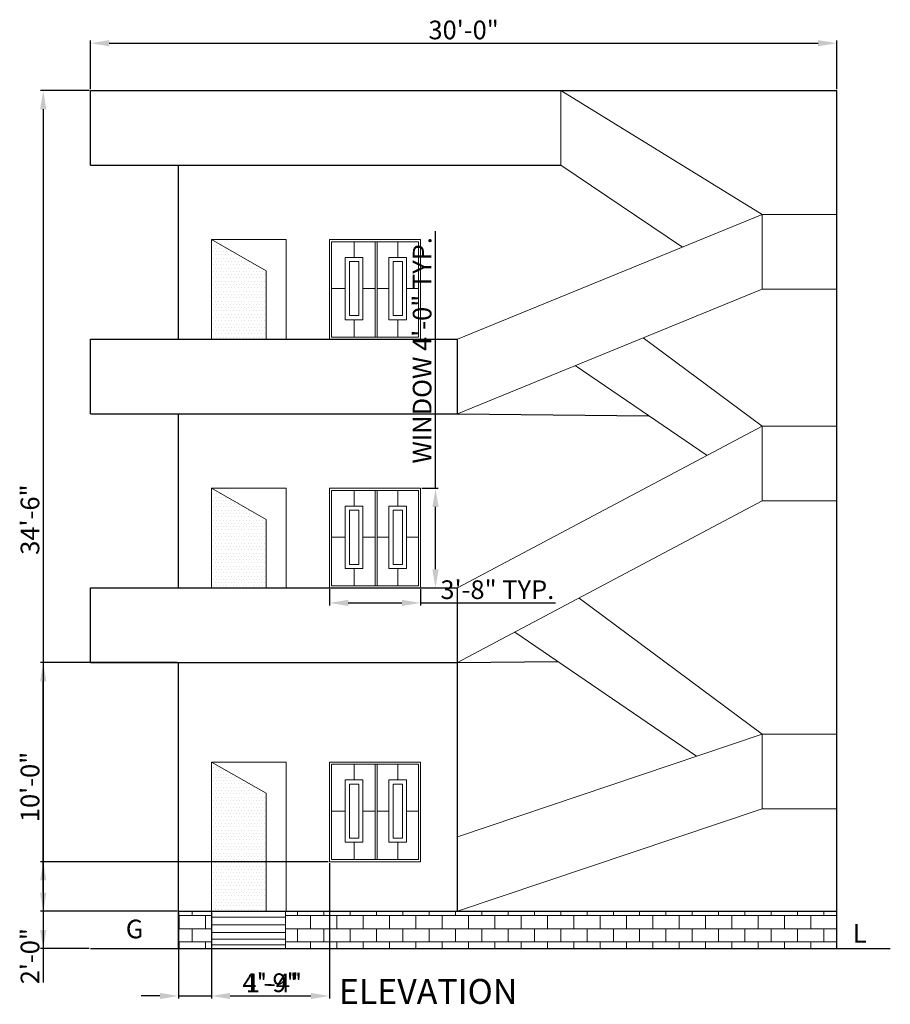
# Model space of a CAD drawing. Units: inches. Extents: x 2044 to 3644, y 808 to 1988.
# Tile 2 of 4: x 2082 to 2502, y 1513 to 1988. Entities that reach past the tile are written whole.
import ezdxf

# ---------------------------------------------------------------- set-up
doc = ezdxf.new("R2010")
doc.units = ezdxf.units.IN
for name, color, linetype, lineweight in [('A-ANNO-DIMS', 2, 'Continuous', 18), ('A-ANNO-SYMB', 2, 'Continuous', 18), ('A-ANNO-TITL', 7, 'Continuous', 25), ('A-DOOR', 4, 'Continuous', 18), ('A-DOOR-PATT', 252, 'Continuous', 13), ('A-ELEV', 7, 'Continuous', 25), ('A-FLOR-STRS', 3, 'Continuous', 18), ('A-GLAZ', 4, 'Continuous', 18), ('A-WALL-PATT', 252, 'Continuous', 13)]:
    doc.layers.add(name, color=color, linetype=linetype, lineweight=lineweight)
doc.styles.get("Standard").update_dxf_attribs({"font": 'arial.ttf'})
doc.dimstyles.new('ISO-25', dxfattribs={"dimtxt": 9, "dimasz": 9, "dimexe": 1.25, "dimexo": 0.625, "dimtad": 1, "dimdec": 1, "dimrnd": 9, "dimlunit": 3, "dimtxsty": 'Standard', "dimcen": 2.5, "dimadec": 0, "dimazin": 0, "dimtfac": 1, "dimtdec": 1, "dimtmove": 0, "dimatfit": 3, "dimfxl": 1, "dimarcsym": 0})

# ---------------------------------------------------------------- blocks, each defined once
blk = doc.blocks.new('WIN-TWIN-PANEL-ELEV')
for p, q in [((11.88, 39.49), (11.88, 47.1)), ((21.96, 47.1), (21.96, 1)), ((22.96, 47.1), (22.96, 1)), ((32.93, 39.49), (32.93, 47.1)), ((1, 24.45), (7.61, 24.45)), ((16.15, 24.45), (21.96, 24.45)), ((22.96, 24.45), (28.66, 24.45)), ((37.2, 24.45), (42.91, 24.45)), ((11.88, 9.41), (11.88, 1)), ((32.93, 9.41), (32.93, 1))]:
    blk.add_line(p, q)
for points in [[(0, 48.1), (43.91, 48.1), (43.91, 0), (0, 0)], [(1, 47.1), (42.91, 47.1), (42.91, 1), (1, 1)], [(7.61, 39.49), (16.15, 39.49), (16.15, 9.41), (7.61, 9.41)], [(28.66, 39.49), (37.2, 39.49), (37.2, 9.41), (28.66, 9.41)], [(9.61, 37.49), (14.15, 37.49), (14.15, 11.41), (9.61, 11.41)], [(30.66, 37.49), (35.2, 37.49), (35.2, 11.41), (30.66, 11.41)]]:
    blk.add_lwpolyline(points, close=True)
blk = doc.blocks.new('*D43')
at = {"layer": 'A-ANNO-DIMS', "color": 0, "lineweight": -2, "transparency": 16777216}
for p, q in [((2282.74, 1761.93), (2282.74, 1886.07)), ((2276.15, 1761.93), (2283.99, 1761.93)), ((2282.74, 1722.83), (2282.74, 1752.93)), ((2276.15, 1713.83), (2283.99, 1713.83))]:
    blk.add_line(p, q, dxfattribs=at)
at = {"layer": 'A-ANNO-DIMS', "color": 0, "transparency": 16777216}
for points in [[(2281.24, 1752.93), (2284.24, 1752.93), (2282.74, 1761.93)], [(2281.24, 1722.83), (2284.24, 1722.83), (2282.74, 1713.83)]]:
    blk.add_solid(points, dxfattribs=at)
at = {"layer": 'Defpoints', "color": 0, "transparency": 16777216}
for p in [(2275.52, 1761.93), (2282.74, 1761.93), (2275.52, 1713.83)]:
    blk.add_point(p, dxfattribs=at)
at = {"layer": 'A-ANNO-DIMS', "color": 0, "transparency": 16777216, "insert": (2277.46, 1828.5), "char_height": 9, "attachment_point": 5, "rotation": 90}
blk.add_mtext('WINDOW 4\'-0" TYP.', dxfattribs=at)
blk = doc.blocks.new('*D44')
at = {"layer": 'A-ANNO-DIMS', "color": 0, "lineweight": -2, "transparency": 16777216}
for p, q in [((2231.61, 1713.21), (2231.61, 1705.37)), ((2275.52, 1713.21), (2275.52, 1705.37)), ((2240.61, 1706.62), (2266.52, 1706.62)), ((2275.52, 1706.62), (2340.63, 1706.62))]:
    blk.add_line(p, q, dxfattribs=at)
at = {"layer": 'A-ANNO-DIMS', "color": 0, "transparency": 16777216}
for points in [[(2240.61, 1708.12), (2240.61, 1705.12), (2231.61, 1706.62)], [(2266.52, 1708.12), (2266.52, 1705.12), (2275.52, 1706.62)]]:
    blk.add_solid(points, dxfattribs=at)
at = {"layer": 'Defpoints', "color": 0, "transparency": 16777216}
for p in [(2231.61, 1713.83), (2275.52, 1713.83), (2275.52, 1706.62)]:
    blk.add_point(p, dxfattribs=at)
at = {"layer": 'A-ANNO-DIMS', "color": 0, "transparency": 16777216, "insert": (2312.58, 1711.84), "char_height": 9, "attachment_point": 5}
blk.add_mtext('3\'-8" TYP.', dxfattribs=at)
blk = doc.blocks.new('*D62')
at = {"layer": 'A-ANNO-DIMS', "color": 0, "lineweight": -2, "transparency": 16777216}
for p, q in [((2116.33, 1954.46), (2116.33, 1977.93)), ((2125.33, 1976.68), (2467.33, 1976.68)), ((2476.33, 1954.46), (2476.33, 1977.93))]:
    blk.add_line(p, q, dxfattribs=at)
at = {"layer": 'A-ANNO-DIMS', "color": 0, "transparency": 16777216}
for points in [[(2125.33, 1978.18), (2125.33, 1975.18), (2116.33, 1976.68)], [(2467.33, 1978.18), (2467.33, 1975.18), (2476.33, 1976.68)]]:
    blk.add_solid(points, dxfattribs=at)
at = {"layer": 'Defpoints', "color": 0, "transparency": 16777216}
for p in [(2476.33, 1976.68), (2116.33, 1953.83), (2476.33, 1953.83)]:
    blk.add_point(p, dxfattribs=at)
at = {"layer": 'A-ANNO-DIMS', "color": 0, "transparency": 16777216, "insert": (2296.33, 1981.91), "char_height": 9, "attachment_point": 5}
blk.add_mtext('30\'-0"', dxfattribs=at)
blk = doc.blocks.new('*D63')
at = {"layer": 'A-ANNO-DIMS', "color": 0, "lineweight": -2, "transparency": 16777216}
for p, q in [((2115.7, 1953.83), (2092.23, 1953.83)), ((2093.48, 1944.83), (2093.48, 1548.83)), ((2115.7, 1539.83), (2092.23, 1539.83))]:
    blk.add_line(p, q, dxfattribs=at)
at = {"layer": 'A-ANNO-DIMS', "color": 0, "transparency": 16777216}
for points in [[(2091.98, 1944.83), (2094.98, 1944.83), (2093.48, 1953.83)], [(2091.98, 1548.83), (2094.98, 1548.83), (2093.48, 1539.83)]]:
    blk.add_solid(points, dxfattribs=at)
at = {"layer": 'Defpoints', "color": 0, "transparency": 16777216}
for p in [(2116.33, 1953.83), (2093.48, 1539.83), (2116.33, 1539.83)]:
    blk.add_point(p, dxfattribs=at)
at = {"layer": 'A-ANNO-DIMS', "color": 0, "transparency": 16777216, "insert": (2088.25, 1746.83), "char_height": 9, "attachment_point": 5, "rotation": 90}
blk.add_mtext('34\'-6"', dxfattribs=at)
blk = doc.blocks.new('*D64')
at = {"layer": 'A-ANNO-DIMS', "color": 0, "lineweight": -2, "transparency": 16777216}
for p, q in [((2158.74, 1557.21), (2158.74, 1515.73)), ((2174.67, 1557.21), (2174.67, 1515.73)), ((2149.74, 1516.98), (2140.74, 1516.98)), ((2158.74, 1516.98), (2174.67, 1516.98)), ((2183.67, 1516.98), (2217, 1516.98))]:
    blk.add_line(p, q, dxfattribs=at)
at = {"layer": 'A-ANNO-DIMS', "color": 0, "transparency": 16777216}
for points in [[(2149.74, 1518.48), (2149.74, 1515.48), (2158.74, 1516.98)], [(2183.67, 1518.48), (2183.67, 1515.48), (2174.67, 1516.98)]]:
    blk.add_solid(points, dxfattribs=at)
at = {"layer": 'Defpoints', "color": 0, "transparency": 16777216}
for p in [(2158.74, 1557.83), (2174.67, 1557.83), (2174.67, 1516.98)]:
    blk.add_point(p, dxfattribs=at)
at = {"layer": 'A-ANNO-DIMS', "color": 0, "transparency": 16777216, "insert": (2204.84, 1522.13), "char_height": 9, "attachment_point": 5}
blk.add_mtext('1\'-4"', dxfattribs=at)
blk = doc.blocks.new('*D65')
at = {"layer": 'A-ANNO-DIMS', "color": 0, "lineweight": -2, "transparency": 16777216}
for p, q in [((2231.61, 1581.11), (2231.61, 1515.73)), ((2174.67, 1557.21), (2174.67, 1515.73)), ((2183.67, 1516.98), (2222.61, 1516.98))]:
    blk.add_line(p, q, dxfattribs=at)
at = {"layer": 'A-ANNO-DIMS', "color": 0, "transparency": 16777216}
for points in [[(2183.67, 1518.48), (2183.67, 1515.48), (2174.67, 1516.98)], [(2222.61, 1518.48), (2222.61, 1515.48), (2231.61, 1516.98)]]:
    blk.add_solid(points, dxfattribs=at)
at = {"layer": 'Defpoints', "color": 0, "transparency": 16777216}
for p in [(2231.61, 1581.74), (2174.67, 1557.83), (2231.61, 1516.98)]:
    blk.add_point(p, dxfattribs=at)
at = {"layer": 'A-ANNO-DIMS', "color": 0, "transparency": 16777216, "insert": (2203.14, 1522.2), "char_height": 9, "attachment_point": 5}
blk.add_mtext('4\'-9"', dxfattribs=at)
blk = doc.blocks.new('*D66')
at = {"layer": 'A-ANNO-DIMS', "color": 0, "lineweight": -2, "transparency": 16777216}
for p, q in [((2230.99, 1581.74), (2092.23, 1581.74)), ((2093.48, 1572.74), (2093.48, 1566.83)), ((2158.12, 1557.83), (2092.23, 1557.83)), ((2093.48, 1557.83), (2093.48, 1523.51))]:
    blk.add_line(p, q, dxfattribs=at)
at = {"layer": 'A-ANNO-DIMS', "color": 0, "transparency": 16777216}
for points in [[(2091.98, 1572.74), (2094.98, 1572.74), (2093.48, 1581.74)], [(2091.98, 1566.83), (2094.98, 1566.83), (2093.48, 1557.83)]]:
    blk.add_solid(points, dxfattribs=at)
at = {"layer": 'Defpoints', "color": 0, "transparency": 16777216}
for p in [(2231.61, 1581.74), (2093.48, 1557.83), (2158.74, 1557.83)]:
    blk.add_point(p, dxfattribs=at)
at = {"layer": 'A-ANNO-DIMS', "color": 0, "transparency": 16777216, "insert": (2088.26, 1536.17), "char_height": 9, "attachment_point": 5, "rotation": 90}
blk.add_mtext('2\'-0"', dxfattribs=at)
blk = doc.blocks.new('*D67')
at = {"layer": 'A-ANNO-DIMS', "color": 0, "lineweight": -2, "transparency": 16777216}
for p, q in [((2158.12, 1677.83), (2092.23, 1677.83)), ((2093.48, 1566.83), (2093.48, 1668.83)), ((2158.12, 1557.83), (2092.23, 1557.83))]:
    blk.add_line(p, q, dxfattribs=at)
at = {"layer": 'A-ANNO-DIMS', "color": 0, "transparency": 16777216}
for points in [[(2091.98, 1668.83), (2094.98, 1668.83), (2093.48, 1677.83)], [(2091.98, 1566.83), (2094.98, 1566.83), (2093.48, 1557.83)]]:
    blk.add_solid(points, dxfattribs=at)
at = {"layer": 'Defpoints', "color": 0, "transparency": 16777216}
for p in [(2093.48, 1677.83), (2158.74, 1677.83), (2158.74, 1557.83)]:
    blk.add_point(p, dxfattribs=at)
at = {"layer": 'A-ANNO-DIMS', "color": 0, "transparency": 16777216, "insert": (2088.26, 1617.83), "char_height": 9, "attachment_point": 5, "rotation": 90}
blk.add_mtext('10\'-0"', dxfattribs=at)

msp = doc.modelspace()

# ---------------------------------------------------------------- hatches: boundary and pattern name
at = {"layer": 'A-DOOR-PATT'}
h = msp.add_hatch(dxfattribs=at)
h.set_pattern_fill('DOTS', color=256)
h.set_pattern_definition([(0, (9e-13, 252.0964), (0.79375, 1.5875), [0, -1.5875])])
h.paths.add_polyline_path([(2174.67, 1833.83), (2201.07, 1833.83), (2201.07, 1866.86), (2174.67, 1881.93)])
h = msp.add_hatch(dxfattribs=at)
h.set_pattern_fill('DOTS', color=256)
h.set_pattern_definition([(0, (1e-12, 132.0964), (0.79375, 1.5875), [0, -1.5875])])
h.paths.add_polyline_path([(2174.67, 1713.83), (2201.07, 1713.83), (2201.07, 1746.86), (2174.67, 1761.93)])
h = msp.add_hatch(dxfattribs=at)
h.set_pattern_fill('DOTS', color=256)
h.paths.add_polyline_path([(2201.07, 1614.76), (2174.67, 1629.83), (2174.67, 1557.83), (2201.07, 1557.83)])
at = {"layer": 'A-WALL-PATT'}
h = msp.add_hatch(dxfattribs=at)
h.set_pattern_fill('BRICK', color=256)
h.paths.add_polyline_path([(2476.33, 1557.83), (2210.41, 1557.83), (2210.41, 1539.83), (2476.33, 1539.83)])
h.paths.add_polyline_path([(2174.67, 1557.83), (2158.74, 1557.83), (2158.74, 1539.83), (2174.67, 1539.83)])

# ---------------------------------------------------------------- linework, layer by layer
at = {"layer": 'A-DOOR'}
for p, q in [((2174.67, 1833.83), (2174.67, 1881.93)), ((2174.67, 1881.93), (2210.67, 1881.93)), ((2174.67, 1881.93), (2201.07, 1866.86)), ((2210.67, 1881.93), (2210.67, 1833.83)), ((2201.07, 1866.86), (2201.07, 1833.83)), ((2174.67, 1713.83), (2174.67, 1761.93)), ((2174.67, 1761.93), (2210.67, 1761.93)), ((2174.67, 1761.93), (2201.07, 1746.86)), ((2210.67, 1761.93), (2210.67, 1713.83)), ((2201.07, 1746.86), (2201.07, 1713.83)), ((2174.67, 1557.83), (2174.67, 1629.83)), ((2174.67, 1629.83), (2210.67, 1629.83)), ((2174.67, 1629.83), (2201.07, 1614.76)), ((2210.67, 1629.83), (2210.67, 1557.83)), ((2201.07, 1614.76), (2201.07, 1557.83))]:
    msp.add_line(p, q, dxfattribs=at)
at = {"layer": 'A-ELEV'}
for p, q in [((2116.33, 1953.83), (2476.33, 1953.83)), ((2116.33, 1917.83), (2116.33, 1953.83)), ((2476.33, 1539.83), (2476.33, 1953.83)), ((2116.33, 1917.83), (2343.17, 1917.83)), ((2158.74, 1833.83), (2158.74, 1917.83)), ((2116.33, 1833.83), (2293.33, 1833.83)), ((2116.33, 1797.83), (2116.33, 1833.83)), ((2293.33, 1797.83), (2293.33, 1833.83)), ((2116.33, 1797.83), (2293.33, 1797.83)), ((2158.74, 1713.83), (2158.74, 1797.83)), ((2293.33, 1797.83), (2385.61, 1796.96)), ((2116.33, 1713.83), (2293.33, 1713.83)), ((2116.33, 1677.83), (2116.33, 1713.83)), ((2293.33, 1557.83), (2293.33, 1713.83)), ((2116.33, 1677.83), (2293.33, 1677.83)), ((2158.74, 1539.83), (2158.74, 1677.83)), ((2293.33, 1677.83), (2341.84, 1678.31)), ((2158.74, 1557.83), (2476.33, 1557.83)), ((2116.33, 1539.83), (2476.33, 1539.83)), ((2476.33, 1539.83), (2502.19, 1539.83))]:
    msp.add_line(p, q, dxfattribs=at)
at = {"layer": 'A-FLOR-STRS'}
for p, q in [((2440.33, 1894.05), (2343.17, 1953.83)), ((2343.17, 1953.83), (2343.17, 1917.83)), ((2343.17, 1917.83), (2401.97, 1878.33)), ((2293.33, 1833.83), (2440.33, 1894.05)), ((2440.33, 1894.05), (2476.33, 1894.05)), ((2440.33, 1858.05), (2440.33, 1894.05)), ((2293.33, 1797.83), (2440.33, 1858.05)), ((2440.33, 1858.05), (2476.33, 1858.05)), ((2440.33, 1791.83), (2382.92, 1834.53)), ((2350.21, 1821.13), (2413.75, 1777.73)), ((2293.33, 1713.83), (2440.33, 1791.83)), ((2440.33, 1791.83), (2476.33, 1791.83)), ((2440.33, 1755.83), (2440.33, 1791.83)), ((2293.33, 1677.83), (2440.33, 1755.83)), ((2440.33, 1755.83), (2476.33, 1755.83)), ((2440.33, 1643.29), (2352.02, 1708.98)), ((2321.02, 1692.53), (2408.72, 1632.63)), ((2440.33, 1643.29), (2293.33, 1593.7)), ((2440.33, 1607.29), (2440.33, 1643.29)), ((2476.33, 1643.29), (2440.33, 1643.29)), ((2293.33, 1557.83), (2440.33, 1607.29)), ((2476.33, 1607.29), (2440.33, 1607.29)), ((2174.67, 1539.83), (2174.67, 1557.83)), ((2174.67, 1555.06), (2210.41, 1555.06)), ((2210.41, 1539.83), (2210.41, 1557.83)), ((2174.67, 1551.25), (2210.41, 1551.25)), ((2174.67, 1547.62), (2210.41, 1547.62)), ((2174.67, 1544.43), (2210.41, 1544.43)), ((2174.67, 1541.67), (2210.41, 1541.67))]:
    msp.add_line(p, q, dxfattribs=at)

# ---------------------------------------------------------------- block references
at = {"layer": 'A-GLAZ'}
for p in [(2231.61, 1833.83), (2231.61, 1713.83), (2231.61, 1581.74)]:
    msp.add_blockref('WIN-TWIN-PANEL-ELEV', p, dxfattribs=at)

# ---------------------------------------------------------------- texts
at = {"layer": 'A-ANNO-SYMB', "char_height": 9, "attachment_point": 1}
for s, insert in [('G', (2133.33, 1553.79)), ('L', (2484.12, 1551.67))]:
    msp.add_mtext_dynamic_manual_height_columns(s, width=19.1778, gutter_width=12.5, heights=[0], dxfattribs=dict(at, insert=insert))
at = {"layer": 'A-ANNO-TITL', "insert": (2236.11, 1525.16), "char_height": 12, "attachment_point": 1}
msp.add_mtext_dynamic_manual_height_columns('ELEVATION', width=134.103, gutter_width=12.5, heights=[0], dxfattribs=at)

# ---------------------------------------------------------------- dimensions: what is measured, and where the dimension line sits
at = {"layer": 'A-ANNO-DIMS'}
for base, p1, p2, picture, middle in [((2476.33, 1976.68), (2116.33, 1953.83), (2476.33, 1953.83), '*D62', (2296.33, 1981.91)), ((2231.61, 1516.98), (2174.67, 1557.83), (2231.61, 1581.74), '*D65', (2203.14, 1522.2)), ((2174.67, 1516.98), (2158.74, 1557.83), (2174.67, 1557.83), '*D64', (2204.84, 1522.13))]:
    dim = msp.add_linear_dim(base=base, p1=p1, p2=p2, dimstyle='ISO-25', override={"dimdec": 1, "dimlfac": 1, "dimrnd": 0, "dimzin": 1, "dimdsep": 46, "dimlunit": 4, "dimfrac": 2}, dxfattribs=at)
    dim.commit()
    dim.dimension.update_dxf_attribs({"geometry": picture, "text_midpoint": middle})
for base, p1, p2, picture, middle in [((2093.48, 1539.83), (2116.33, 1953.83), (2116.33, 1539.83), '*D63', (2088.25, 1746.83)), ((2093.48, 1677.83), (2158.74, 1557.83), (2158.74, 1677.83), '*D67', (2088.26, 1617.83)), ((2093.48, 1557.83), (2231.61, 1581.74), (2158.74, 1557.83), '*D66', (2088.26, 1536.17))]:
    dim = msp.add_linear_dim(base=base, p1=p1, p2=p2, angle=90, dimstyle='ISO-25', override={"dimdec": 1, "dimlfac": 1, "dimrnd": 0, "dimzin": 1, "dimdsep": 46, "dimlunit": 4, "dimfrac": 2}, dxfattribs=at)
    dim.commit()
    dim.dimension.update_dxf_attribs({"geometry": picture, "text_midpoint": middle})
dim = msp.add_linear_dim(base=(2282.74, 1761.93), p1=(2275.52, 1713.83), p2=(2275.52, 1761.93), angle=90, text='WINDOW <> TYP.', dimstyle='ISO-25', override={"dimdec": 1, "dimlfac": 1, "dimrnd": 0, "dimzin": 1, "dimdsep": 46, "dimlunit": 4, "dimfrac": 2}, dxfattribs=at)
dim.commit()
dim.dimension.update_dxf_attribs({"geometry": '*D43', "text_midpoint": (2277.46, 1828.5)})
dim = msp.add_linear_dim(base=(2275.52, 1706.62), p1=(2231.61, 1713.83), p2=(2275.52, 1713.83), text='<> TYP.', dimstyle='ISO-25', override={"dimdec": 1, "dimlfac": 1, "dimrnd": 0, "dimzin": 1, "dimdsep": 46, "dimlunit": 4, "dimfrac": 2}, dxfattribs=at)
dim.commit()
dim.dimension.update_dxf_attribs({"geometry": '*D44', "text_midpoint": (2312.58, 1711.84)})

doc.saveas('drawing.dxf')
